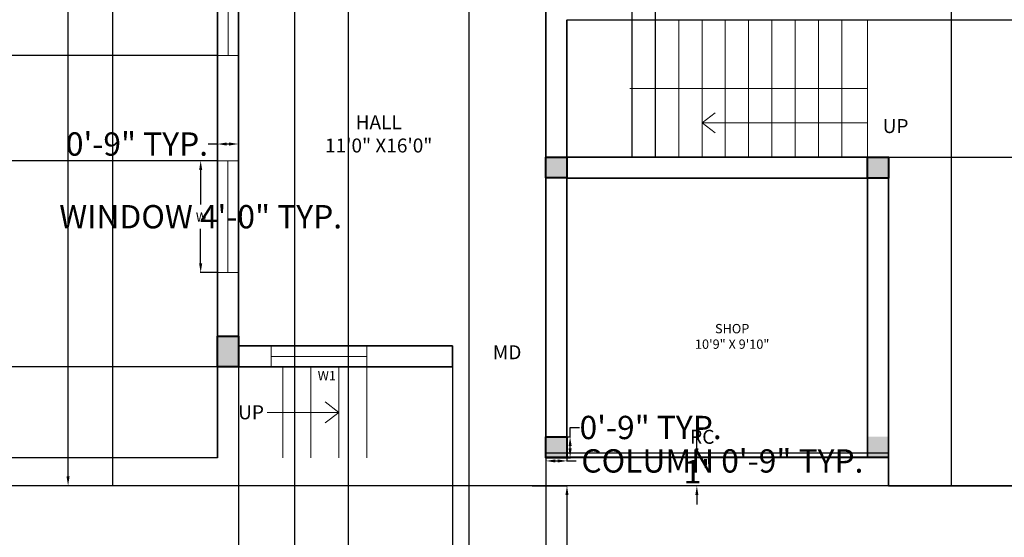
# Model space of a CAD drawing. Units: inches. Extents: x 529 to 1659, y 271 to 1222.
# Tile 3 of 5: x 936 to 1358, y 664 to 886. Entities that reach past the tile are written whole.
import ezdxf

# ---------------------------------------------------------------- set-up
doc = ezdxf.new("R2010")
doc.units = ezdxf.units.IN
doc.header["$MEASUREMENT"] = 0
for name, color, linetype, lineweight in [('A-AREA-IDEN', 7, 'Continuous', 18), ('A-COLS', 7, 'Continuous', 40), ('A-COLS-PATT', 252, 'Continuous', 13), ('A-DOOR-PATT', 4, 'Continuous', 13), ('C-ROAD', 7, 'Continuous', 25), ('COMPOUND WALL', 7, 'Continuous', 25), ('DIM', 241, 'Continuous', 18), ('DOOR', 4, 'Continuous', 25), ('STAIRCASE', 132, 'Continuous', 18), ('TEXT', 131, 'Continuous', 18), ('WALL', 7, 'Continuous', 35), ('WDS', 4, 'Continuous', 18)]:
    doc.layers.add(name, color=color, linetype=linetype, lineweight=lineweight)
doc.styles.get("Standard").update_dxf_attribs({"font": 'arial.ttf', "height": 10})
doc.dimstyles.get("Standard").update_dxf_attribs({"dimtxt": 6, "dimasz": 4, "dimexe": 0.18, "dimexo": 0.0625, "dimgap": 0.09, "dimtad": 0, "dimtih": 1, "dimtoh": 1, "dimdec": 0, "dimrnd": 6, "dimzin": 0, "dimdsep": 46, "dimlunit": 3, "dimtxsty": 'Standard', "dimcen": 0.09, "dimadec": 0, "dimazin": 0, "dimtfac": 1, "dimtdec": 0, "dimtofl": 0, "dimtmove": 0, "dimatfit": 3, "dimfxl": 1, "dimtolj": 1, "dimtzin": 0, "dimarcsym": 0})

# ---------------------------------------------------------------- blocks, each defined once
blk = doc.blocks.new('*D4')
at = {"layer": 'Defpoints', "color": 0, "transparency": 16777216}
for p in [(1228.33, 697.86), (1226.27, 685.86), (1228.33, 685.86)]:
    blk.add_point(p, dxfattribs=at)
at = {"layer": 'DIM', "color": 0, "lineweight": -2, "transparency": 16777216}
for p, q in [((1226.27, 701.86), (1226.27, 705.86)), ((1228.26, 697.86), (1226.09, 697.86)), ((1228.26, 685.86), (1226.09, 685.86)), ((1226.27, 681.86), (1226.27, 677.86))]:
    blk.add_line(p, q, dxfattribs=at)
at = {"layer": 'DIM', "color": 0, "transparency": 16777216}
for points in [[(1225.6, 701.86), (1226.94, 701.86), (1226.27, 697.86)], [(1225.6, 681.86), (1226.94, 681.86), (1226.27, 685.86)]]:
    blk.add_solid(points, dxfattribs=at)
at = {"layer": 'DIM', "color": 0, "transparency": 16777216, "insert": (1226.27, 691.86), "char_height": 10, "attachment_point": 5}
blk.add_mtext("\\A1;1'", dxfattribs=at)
blk = doc.blocks.new('*D5')
at = {"layer": 'Defpoints', "color": 0, "transparency": 16777216}
for p in [(956.28, 1165.86), (975.49, 1165.86), (975.49, 685.86)]:
    blk.add_point(p, dxfattribs=at)
at = {"layer": 'DIM', "color": 0, "lineweight": -2, "transparency": 16777216}
for p, q in [((975.43, 1165.86), (956.1, 1165.86)), ((956.28, 1161.86), (956.28, 931.05)), ((956.28, 689.86), (956.28, 920.66)), ((975.43, 685.86), (956.1, 685.86))]:
    blk.add_line(p, q, dxfattribs=at)
at = {"layer": 'DIM', "color": 0, "transparency": 16777216}
for points in [[(955.61, 1161.86), (956.94, 1161.86), (956.28, 1165.86)], [(955.61, 689.86), (956.94, 689.86), (956.28, 685.86)]]:
    blk.add_solid(points, dxfattribs=at)
at = {"layer": 'DIM', "color": 0, "transparency": 16777216, "insert": (956.28, 925.86), "char_height": 10, "attachment_point": 5}
blk.add_mtext("\\A1;40'", dxfattribs=at)
blk = doc.blocks.new('*D8')
at = {"layer": 'Defpoints', "color": 0, "transparency": 16777216}
for p in [(1155.49, 685.86), (1170.49, 685.86), (1155.55, 327.24)]:
    blk.add_point(p, dxfattribs=at)
at = {"layer": 'DIM', "color": 0, "lineweight": -2, "transparency": 16777216}
for p, q in [((1155.56, 685.86), (1170.67, 685.86)), ((1170.49, 681.86), (1170.49, 511.75)), ((1170.49, 331.24), (1170.49, 501.35)), ((1155.61, 327.24), (1170.67, 327.24))]:
    blk.add_line(p, q, dxfattribs=at)
at = {"layer": 'DIM', "color": 0, "transparency": 16777216}
for points in [[(1169.83, 681.86), (1171.16, 681.86), (1170.49, 685.86)], [(1169.83, 331.24), (1171.16, 331.24), (1170.49, 327.24)]]:
    blk.add_solid(points, dxfattribs=at)
at = {"layer": 'DIM', "color": 0, "transparency": 16777216, "insert": (1170.49, 506.55), "char_height": 10, "attachment_point": 5}
blk.add_mtext("\\A1;30'", dxfattribs=at)
blk = doc.blocks.new('WIN-48IN')
for p, q in [((9, 48), (0, 48)), ((4.5, 0), (4.5, 48)), ((9, 0), (0, 0))]:
    blk.add_line(p, q)
blk = doc.blocks.new('COL-9X9IN')
blk.add_lwpolyline([(0, 9), (9, 9), (9, 0), (0, 0)], close=True)
blk = doc.blocks.new('*D17')
at = {"layer": 'Defpoints', "color": 0, "transparency": 16777216}
for p in [(1161.49, 697.86), (1170.49, 697.86), (1170.49, 696.51)]:
    blk.add_point(p, dxfattribs=at)
at = {"layer": 'DIM', "color": 0, "lineweight": -2, "transparency": 16777216}
for p, q in [((1161.49, 697.79), (1161.49, 696.33)), ((1170.49, 697.79), (1170.49, 696.33)), ((1165.49, 696.51), (1166.49, 696.51)), ((1170.49, 696.51), (1174.49, 696.51))]:
    blk.add_line(p, q, dxfattribs=at)
at = {"layer": 'DIM', "color": 0, "transparency": 16777216}
for points in [[(1165.49, 697.17), (1165.49, 695.84), (1161.49, 696.51)], [(1166.49, 697.17), (1166.49, 695.84), (1170.49, 696.51)]]:
    blk.add_solid(points, dxfattribs=at)
at = {"layer": 'DIM', "color": 0, "transparency": 16777216, "insert": (1237.21, 696.51), "char_height": 10, "attachment_point": 5}
blk.add_mtext('\\A1;COLUMN 0\'-9" TYP.', dxfattribs=at)
blk = doc.blocks.new('*D18')
at = {"layer": 'Defpoints', "color": 0, "transparency": 16777216}
for p in [(1170.49, 706.86), (1171.84, 706.86), (1170.49, 697.86)]:
    blk.add_point(p, dxfattribs=at)
at = {"layer": 'DIM', "color": 0, "lineweight": -2, "transparency": 16777216}
for p, q in [((1171.84, 706.86), (1171.84, 710.86)), ((1171.84, 710.86), (1175.84, 710.86)), ((1170.56, 706.86), (1172.02, 706.86)), ((1171.84, 701.86), (1171.84, 702.86)), ((1170.56, 697.86), (1172.02, 697.86))]:
    blk.add_line(p, q, dxfattribs=at)
at = {"layer": 'DIM', "color": 0, "transparency": 16777216}
for points in [[(1171.18, 702.86), (1172.51, 702.86), (1171.84, 706.86)], [(1171.18, 701.86), (1172.51, 701.86), (1171.84, 697.86)]]:
    blk.add_solid(points, dxfattribs=at)
at = {"layer": 'DIM', "color": 0, "transparency": 16777216, "insert": (1206.41, 710.86), "char_height": 10, "attachment_point": 5}
blk.add_mtext('\\A1;0\'-9" TYP.', dxfattribs=at)
blk = doc.blocks.new('*D21')
at = {"layer": 'Defpoints', "color": 0, "transparency": 16777216}
for p in [(1020.41, 825.31), (1013.21, 777.31), (1020.41, 777.31)]:
    blk.add_point(p, dxfattribs=at)
at = {"layer": 'DIM', "color": 0, "lineweight": -2, "transparency": 16777216}
for p, q in [((1020.35, 825.31), (1013.03, 825.31)), ((1013.21, 821.31), (1013.21, 806.57)), ((1013.21, 781.31), (1013.21, 796.04)), ((1020.35, 777.31), (1013.03, 777.31))]:
    blk.add_line(p, q, dxfattribs=at)
at = {"layer": 'DIM', "color": 0, "transparency": 16777216}
for points in [[(1012.55, 821.31), (1013.88, 821.31), (1013.21, 825.31)], [(1012.55, 781.31), (1013.88, 781.31), (1013.21, 777.31)]]:
    blk.add_solid(points, dxfattribs=at)
at = {"layer": 'DIM', "color": 0, "transparency": 16777216, "insert": (1013.21, 801.31), "char_height": 10, "attachment_point": 5}
blk.add_mtext('\\A1;WINDOW 4\'-0" TYP.', dxfattribs=at)
blk = doc.blocks.new('*D22')
at = {"layer": 'Defpoints', "color": 0, "transparency": 16777216}
for p in [(1020.41, 832.51), (1020.41, 825.31), (1029.41, 825.31)]:
    blk.add_point(p, dxfattribs=at)
at = {"layer": 'DIM', "color": 0, "lineweight": -2, "transparency": 16777216}
for p, q in [((1020.41, 832.51), (1016.41, 832.51)), ((1020.41, 825.37), (1020.41, 832.69)), ((1025.41, 832.51), (1024.41, 832.51)), ((1029.41, 825.37), (1029.41, 832.69))]:
    blk.add_line(p, q, dxfattribs=at)
at = {"layer": 'DIM', "color": 0, "transparency": 16777216}
for points in [[(1024.41, 833.17), (1024.41, 831.84), (1020.41, 832.51)], [(1025.41, 833.17), (1025.41, 831.84), (1029.41, 832.51)]]:
    blk.add_solid(points, dxfattribs=at)
at = {"layer": 'DIM', "color": 0, "transparency": 16777216, "insert": (985.85, 832.51), "char_height": 10, "attachment_point": 5}
blk.add_mtext('\\A1;0\'-9" TYP.', dxfattribs=at)
blk = doc.blocks.new('*D28')
at = {"layer": 'Defpoints', "color": 0, "transparency": 16777216}
for p in [(1308.49, 1135.86), (1630, 1135.86), (1308.49, 685.86)]:
    blk.add_point(p, dxfattribs=at)
at = {"layer": 'DIM', "color": 0, "lineweight": -2, "transparency": 16777216}
for p, q in [((1308.56, 1135.86), (1630.18, 1135.86)), ((1630, 1131.86), (1630, 916.05)), ((1630, 689.86), (1630, 905.66)), ((1308.56, 685.86), (1630.18, 685.86))]:
    blk.add_line(p, q, dxfattribs=at)
at = {"layer": 'DIM', "color": 0, "transparency": 16777216}
for points in [[(1629.34, 1131.86), (1630.67, 1131.86), (1630, 1135.86)], [(1629.34, 689.86), (1630.67, 689.86), (1630, 685.86)]]:
    blk.add_solid(points, dxfattribs=at)
at = {"layer": 'DIM', "color": 0, "transparency": 16777216, "insert": (1630, 910.86), "char_height": 10, "attachment_point": 5}
blk.add_mtext('\\A1;37\'-6"', dxfattribs=at)
blk = doc.blocks.new('*D29')
at = {"layer": 'Defpoints', "color": 0, "transparency": 16777216}
for p in [(1076.49, 941.86), (1128.41, 941.86), (1128.41, 277.14)]:
    blk.add_point(p, dxfattribs=at)
at = {"layer": 'DIM', "color": 0, "lineweight": -2, "transparency": 16777216}
for p, q in [((1076.49, 941.79), (1076.49, 276.96)), ((1128.41, 941.79), (1128.41, 276.96)), ((1080.49, 277.14), (1088.87, 277.14)), ((1124.41, 277.14), (1116.04, 277.14))]:
    blk.add_line(p, q, dxfattribs=at)
at = {"layer": 'DIM', "color": 0, "transparency": 16777216}
for points in [[(1080.49, 277.81), (1080.49, 276.47), (1076.49, 277.14)], [(1124.41, 277.81), (1124.41, 276.47), (1128.41, 277.14)]]:
    blk.add_solid(points, dxfattribs=at)
at = {"layer": 'DIM', "color": 0, "transparency": 16777216, "insert": (1102.45, 277.14), "char_height": 10, "attachment_point": 5}
blk.add_mtext('\\A1;4\'-4"', dxfattribs=at)
blk = doc.blocks.new('*D30')
at = {"layer": 'Defpoints', "color": 0, "transparency": 16777216}
for p in [(1170.49, 885.86), (1630, 885.86), (1170.49, 826.86)]:
    blk.add_point(p, dxfattribs=at)
at = {"layer": 'DIM', "color": 0, "lineweight": -2, "transparency": 16777216}
for p, q in [((1170.56, 885.86), (1630.18, 885.86)), ((1630, 881.86), (1630, 861.47)), ((1630, 830.86), (1630, 851.24)), ((1170.56, 826.86), (1630.18, 826.86))]:
    blk.add_line(p, q, dxfattribs=at)
at = {"layer": 'DIM', "color": 0, "transparency": 16777216}
for points in [[(1629.34, 881.86), (1630.67, 881.86), (1630, 885.86)], [(1629.34, 830.86), (1630.67, 830.86), (1630, 826.86)]]:
    blk.add_solid(points, dxfattribs=at)
at = {"layer": 'DIM', "color": 0, "transparency": 16777216, "insert": (1630, 856.36), "char_height": 10, "attachment_point": 5}
blk.add_mtext('\\A1;4\'-11"', dxfattribs=at)
blk = doc.blocks.new('*D31')
at = {"layer": 'Defpoints', "color": 0, "transparency": 16777216}
for p in [(1121.32, 736.86), (1161.49, 736.86), (1161.49, 277.14)]:
    blk.add_point(p, dxfattribs=at)
at = {"layer": 'DIM', "color": 0, "lineweight": -2, "transparency": 16777216}
for p, q in [((1121.32, 736.79), (1121.32, 276.96)), ((1161.49, 736.79), (1161.49, 276.96)), ((1125.32, 277.14), (1128.03, 277.14)), ((1157.49, 277.14), (1154.78, 277.14))]:
    blk.add_line(p, q, dxfattribs=at)
at = {"layer": 'DIM', "color": 0, "transparency": 16777216}
for points in [[(1125.32, 277.81), (1125.32, 276.47), (1121.32, 277.14)], [(1157.49, 277.81), (1157.49, 276.47), (1161.49, 277.14)]]:
    blk.add_solid(points, dxfattribs=at)
at = {"layer": 'DIM', "color": 0, "transparency": 16777216, "insert": (1141.41, 277.14), "char_height": 10, "attachment_point": 5}
blk.add_mtext('\\A1;3\'-4"', dxfattribs=at)
blk = doc.blocks.new('*D32')
at = {"layer": 'Defpoints', "color": 0, "transparency": 16777216}
for p in [(555.49, 736.86), (1020.49, 736.86), (1020.49, 697.86)]:
    blk.add_point(p, dxfattribs=at)
at = {"layer": 'DIM', "color": 0, "lineweight": -2, "transparency": 16777216}
for p, q in [((1020.43, 736.86), (555.31, 736.86)), ((555.49, 732.86), (555.49, 722.55)), ((555.49, 701.86), (555.49, 712.16)), ((1020.43, 697.86), (555.31, 697.86))]:
    blk.add_line(p, q, dxfattribs=at)
at = {"layer": 'DIM', "color": 0, "transparency": 16777216}
for points in [[(554.83, 732.86), (556.16, 732.86), (555.49, 736.86)], [(554.83, 701.86), (556.16, 701.86), (555.49, 697.86)]]:
    blk.add_solid(points, dxfattribs=at)
at = {"layer": 'DIM', "color": 0, "transparency": 16777216, "insert": (555.49, 717.36), "char_height": 10, "attachment_point": 5}
blk.add_mtext('\\A1;3\'-3"', dxfattribs=at)
blk = doc.blocks.new('*D33')
at = {"layer": 'Defpoints', "color": 0, "transparency": 16777216}
for p in [(555.49, 870.44), (1020.49, 870.44), (1020.41, 825.31)]:
    blk.add_point(p, dxfattribs=at)
at = {"layer": 'DIM', "color": 0, "lineweight": -2, "transparency": 16777216}
for p, q in [((1020.43, 870.44), (555.31, 870.44)), ((555.49, 866.44), (555.49, 853.07)), ((555.49, 829.31), (555.49, 842.67)), ((1020.35, 825.31), (555.31, 825.31))]:
    blk.add_line(p, q, dxfattribs=at)
at = {"layer": 'DIM', "color": 0, "transparency": 16777216}
for points in [[(554.83, 866.44), (556.16, 866.44), (555.49, 870.44)], [(554.83, 829.31), (556.16, 829.31), (555.49, 825.31)]]:
    blk.add_solid(points, dxfattribs=at)
at = {"layer": 'DIM', "color": 0, "transparency": 16777216, "insert": (555.49, 847.87), "char_height": 10, "attachment_point": 5}
blk.add_mtext('\\A1;3\'-9"', dxfattribs=at)
blk = doc.blocks.new('*D36')
at = {"layer": 'Defpoints', "color": 0, "transparency": 16777216}
for p in [(1029.49, 1126.86), (1053.49, 1102.86), (1053.49, 277.14)]:
    blk.add_point(p, dxfattribs=at)
at = {"layer": 'DIM', "color": 0, "lineweight": -2, "transparency": 16777216}
for p, q in [((1029.49, 1126.79), (1029.49, 276.96)), ((1053.49, 1102.79), (1053.49, 276.96)), ((1033.49, 277.14), (1049.49, 277.14)), ((1053.49, 277.14), (1057.49, 277.14))]:
    blk.add_line(p, q, dxfattribs=at)
at = {"layer": 'DIM', "color": 0, "transparency": 16777216}
for points in [[(1033.49, 277.81), (1033.49, 276.47), (1029.49, 277.14)], [(1049.49, 277.81), (1049.49, 276.47), (1053.49, 277.14)]]:
    blk.add_solid(points, dxfattribs=at)
at = {"layer": 'DIM', "color": 0, "transparency": 16777216, "insert": (1070.96, 277.14), "char_height": 10, "attachment_point": 5}
blk.add_mtext('\\A1;2\'-0"', dxfattribs=at)
blk = doc.blocks.new('*D37')
at = {"layer": 'Defpoints', "color": 0, "transparency": 16777216}
for p in [(1208.47, 1214.96), (1198.47, 826.86), (1208.47, 826.86)]:
    blk.add_point(p, dxfattribs=at)
at = {"layer": 'DIM', "color": 0, "lineweight": -2, "transparency": 16777216}
for p, q in [((1198.47, 826.92), (1198.47, 1215.14)), ((1202.47, 1214.96), (1204.47, 1214.96)), ((1208.47, 826.92), (1208.47, 1215.14)), ((1208.47, 1214.96), (1212.47, 1214.96))]:
    blk.add_line(p, q, dxfattribs=at)
at = {"layer": 'DIM', "color": 0, "transparency": 16777216}
for points in [[(1202.47, 1215.62), (1202.47, 1214.29), (1198.47, 1214.96)], [(1204.47, 1215.62), (1204.47, 1214.29), (1208.47, 1214.96)]]:
    blk.add_solid(points, dxfattribs=at)
at = {"layer": 'DIM', "color": 0, "transparency": 16777216, "insert": (1229.74, 1214.96), "char_height": 10, "attachment_point": 5}
blk.add_mtext('\\A1;0\'-10"', dxfattribs=at)

msp = doc.modelspace()

# ---------------------------------------------------------------- hatches: boundary and pattern name
at = {"layer": 'A-COLS-PATT'}
h = msp.add_hatch(color=256, dxfattribs=at)
h.dxf.hatch_style = 1
h.paths.add_polyline_path([(1169.49, 1135.86), (1159.82, 1135.86), (1159.82, 1125.57), (1169.49, 1125.57), (1169.49, 1126.86)])
h.paths.add_polyline_path([(1308.49, 1135.86), (1299.49, 1135.86), (1299.49, 1126.86), (1308.49, 1126.86)])
h.paths.add_polyline_path([(1029.49, 1135.86), (1020.49, 1135.86), (1020.49, 1122.62), (1029.49, 1122.62)])
h.paths.add_polyline_path([(1029.49, 941.86), (1020.49, 941.86), (1020.49, 931.16), (1029.49, 931.16)])
h.paths.add_polyline_path([(1170.49, 941.72), (1161.49, 941.72), (1161.49, 932.72), (1170.49, 932.72)])
h.paths.add_polyline_path([(1308.49, 941.86), (1299.49, 941.86), (1299.49, 928.64), (1308.49, 928.64)])
h.paths.add_polyline_path([(1308.49, 826.86), (1299.49, 826.86), (1299.49, 817.86), (1308.49, 817.86)])
h.paths.add_polyline_path([(1170.49, 826.93), (1161.49, 826.93), (1161.49, 817.93), (1170.49, 817.93)])
h.paths.add_polyline_path([(1308.49, 706.86), (1299.49, 706.86), (1299.49, 697.86), (1308.49, 697.86)])
h.paths.add_polyline_path([(1170.49, 706.86), (1161.49, 706.86), (1161.49, 697.86), (1170.49, 697.86)])
h.paths.add_polyline_path([(1029.41, 750.01), (1020.49, 750.01), (1020.49, 736.86), (1029.49, 736.86)])
at = {"layer": 'A-DOOR-PATT'}
h = msp.add_hatch(dxfattribs=at)
h.set_pattern_fill('ANSI31', color=256, scale=0.8, angle=-45, style=0)
h.paths.add_polyline_path([(1161.49, 697.86), (1308.49, 697.86), (1308.49, 698.36), (1161.49, 698.36)])

# ---------------------------------------------------------------- linework, layer by layer
at = {"layer": 'A-COLS'}
for p, q in [((1020.41, 750.01), (1029.41, 750.01)), ((1020.49, 736.86), (1020.41, 750.01)), ((1029.41, 750.01), (1029.49, 736.86)), ((1029.49, 736.86), (1020.49, 736.86))]:
    msp.add_line(p, q, dxfattribs=at)
at = {"layer": 'C-ROAD'}
msp.add_line((1567.16, 685.86), (618.33, 685.86), dxfattribs=at)
msp.add_line((1567.16, 685.86), (618.33, 685.86), dxfattribs=at)
at = {"layer": 'COMPOUND WALL'}
for p, q in [((975.49, 685.86), (975.49, 1165.86)), ((1335.49, 1165.86), (1335.49, 685.86)), ((1335.49, 685.86), (975.49, 685.86))]:
    msp.add_line(p, q, dxfattribs=at)
at = {"layer": 'DOOR'}
for p, q in [((1308.49, 699.86), (1161.49, 699.86)), ((1161.49, 697.86), (1161.49, 698.36))]:
    msp.add_line(p, q, dxfattribs=at)
at = {"layer": 'STAIRCASE'}
for p, q in [((1198.47, 885.86), (1198.47, 826.86)), ((1208.47, 885.86), (1208.47, 826.86)), ((1218.48, 885.86), (1218.48, 826.86)), ((1228.48, 885.86), (1228.48, 826.86)), ((1238.48, 885.86), (1238.48, 826.86)), ((1248.48, 885.86), (1248.48, 826.86)), ((1258.49, 885.86), (1258.49, 826.86)), ((1268.49, 885.86), (1268.49, 826.86)), ((1278.49, 885.86), (1278.49, 826.86)), ((1288.49, 885.86), (1288.49, 826.86)), ((1299.49, 885.86), (1299.49, 826.86)), ((1299.49, 856.36), (1197.47, 856.36)), ((1228.48, 841.61), (1234.14, 845.92)), ((1299.49, 841.61), (1228.48, 841.61)), ((1228.48, 841.61), (1234.14, 837.29)), ((1048.49, 697.86), (1048.49, 736.86)), ((1060.49, 697.86), (1060.49, 736.86)), ((1072.49, 697.86), (1072.49, 736.86)), ((1084.49, 697.86), (1084.49, 736.86)), ((1072.49, 717.36), (1066.69, 721.89)), ((1041.72, 717.36), (1072.49, 717.36)), ((1072.49, 717.36), (1066.69, 712.82))]:
    msp.add_line(p, q, dxfattribs=at)
at = {"layer": 'WALL'}
for p, q in [((1020.49, 697.86), (1020.49, 1135.86)), ((1029.49, 736.86), (1029.49, 980.86)), ((1161.49, 736.86), (1161.49, 941.86)), ((1170.49, 826.86), (1170.49, 885.86)), ((1308.49, 826.86), (1170.49, 826.86)), ((1308.49, 826.86), (1308.49, 685.86)), ((1308.49, 826.86), (1308.49, 685.86)), ((1170.49, 697.86), (1170.49, 817.86)), ((1299.49, 817.86), (1170.49, 817.86)), ((1299.49, 817.86), (1299.49, 697.86)), ((1029.49, 745.86), (1121.32, 745.86)), ((1121.32, 736.86), (1121.32, 745.86)), ((1020.49, 736.86), (1121.32, 736.86)), ((1161.49, 697.86), (1161.49, 736.86))]:
    msp.add_line(p, q, dxfattribs=at)
at = {"layer": 'WDS'}
for p, q in [((1043.5, 736.86), (1043.5, 745.86)), ((1084.49, 736.86), (1084.49, 745.86)), ((1084.49, 741.36), (1043.5, 741.36))]:
    msp.add_line(p, q, dxfattribs=at)

# ---------------------------------------------------------------- block references
at = {"layer": 'A-COLS'}
for p in [(1161.49, 817.93), (1299.49, 817.85), (1161.49, 697.86)]:
    msp.add_blockref('COL-9X9IN', p, dxfattribs=at)
at = {"layer": 'WDS'}
msp.add_blockref('WIN-48IN', (1020.49, 870.43), dxfattribs=at)
at = {"layer": 'WDS', "rotation": 180}
msp.add_blockref('WIN-48IN', (1029.41, 825.31), dxfattribs=at)

# ---------------------------------------------------------------- texts
at = {"layer": 'A-AREA-IDEN', "attachment_point": 1}
for s, width, insert, char_height in [('\\pxqc;HALL\\P11\'0" X16\'0"', 59.3536, (1059.97, 844.87), 6), ('\\pxqc;SHOP\\P10\'9" X 9\'10"', 41.7934, (1220.53, 755.28), 4)]:
    msp.add_mtext_dynamic_manual_height_columns(s, width=width, gutter_width=20, heights=[0], dxfattribs=dict(at, insert=insert, char_height=char_height))
at = {"layer": 'TEXT', "attachment_point": 1}
for s, width, gutter_width, insert, char_height in [('\\pxqc;UP', 16.0307, 20, (1303.57, 843.22), 6), ('W ', 22.0133, 20, (1011.14, 803.17), 4), ('\\pxqc;MD', 21.6865, 20, (1133.96, 746.13), 6), ('W1 ', 22.0133, 20, (1063.46, 735.06), 4), ('\\pxqc;UP', 12.7261, 20, (1028.48, 720.37), 6), ('RC', 37.456, 50, (1223.38, 709.86), 6)]:
    msp.add_mtext_dynamic_manual_height_columns(s, width=width, gutter_width=gutter_width, heights=[0], dxfattribs=dict(at, insert=insert, char_height=char_height))

# ---------------------------------------------------------------- dimensions: what is measured, and where the dimension line sits
at = {"layer": 'DIM'}
for base, p1, p2, picture, middle in [((1208.47, 1214.96), (1198.47, 826.86), (1208.47, 826.86), '*D37', (1229.74, 1214.96)), ((1053.49, 277.14), (1029.49, 1126.86), (1053.49, 1102.86), '*D36', (1070.96, 277.14)), ((1128.41, 277.14), (1076.49, 941.86), (1128.41, 941.86), '*D29', (1102.45, 277.14)), ((1161.49, 277.14), (1121.32, 736.86), (1161.49, 736.86), '*D31', (1141.41, 277.14))]:
    dim = msp.add_linear_dim(base=base, p1=p1, p2=p2, dimstyle='Standard', override={"dimdec": 1, "dimlfac": 1, "dimrnd": 0, "dimzin": 1, "dimdsep": 46, "dimlunit": 4, "dimfrac": 2}, dxfattribs=at)
    dim.commit()
    dim.dimension.update_dxf_attribs({"geometry": picture, "text_midpoint": middle})
for base, p1, p2, override, picture, middle in [((956.28, 1165.86), (975.49, 685.86), (975.49, 1165.86), {"dimclrd": 0, "dimclre": 0, "dimclrt": 0}, '*D5', (956.28, 925.86)), ((1630, 1135.86), (1308.49, 685.86), (1308.49, 1135.86), {"dimdec": 1, "dimlfac": 1, "dimrnd": 0, "dimzin": 1, "dimdsep": 46, "dimlunit": 4, "dimfrac": 2}, '*D28', (1630, 910.86)), ((1630, 885.86), (1170.49, 826.86), (1170.49, 885.86), {"dimdec": 1, "dimlfac": 1, "dimrnd": 0, "dimzin": 1, "dimdsep": 46, "dimlunit": 4, "dimfrac": 2}, '*D30', (1630, 856.36)), ((555.49, 870.44), (1020.41, 825.31), (1020.49, 870.44), {"dimdec": 1, "dimlfac": 1, "dimrnd": 0, "dimzin": 1, "dimdsep": 46, "dimlunit": 4, "dimfrac": 2}, '*D33', (555.49, 847.87)), ((555.49, 736.86), (1020.49, 697.86), (1020.49, 736.86), {"dimdec": 1, "dimlfac": 1, "dimrnd": 0, "dimzin": 1, "dimdsep": 46, "dimlunit": 4, "dimfrac": 2}, '*D32', (555.49, 717.36)), ((1226.27, 685.86), (1228.33, 697.86), (1228.33, 685.86), {"dimclrd": 0, "dimclre": 0, "dimclrt": 0}, '*D4', (1226.27, 691.86)), ((1170.49, 685.86), (1155.55, 327.24), (1155.49, 685.86), {"dimclrd": 0, "dimclre": 0, "dimclrt": 0}, '*D8', (1170.49, 506.55))]:
    dim = msp.add_linear_dim(base=base, p1=p1, p2=p2, angle=90, dimstyle='Standard', override=override, dxfattribs=at)
    dim.commit()
    dim.dimension.update_dxf_attribs({"geometry": picture, "text_midpoint": middle})
for base, p1, p2, angle, text, picture, middle in [((1020.41, 832.51), (1029.41, 825.31), (1020.41, 825.31), 180, '<> TYP.', '*D22', (985.85, 832.51)), ((1013.21, 777.31), (1020.41, 825.31), (1020.41, 777.31), 270, 'WINDOW <> TYP.', '*D21', (1013.21, 801.31)), ((1171.84, 706.86), (1170.49, 697.86), (1170.49, 706.86), 90, '<> TYP.', '*D18', (1206.41, 710.86))]:
    dim = msp.add_linear_dim(base=base, p1=p1, p2=p2, angle=angle, text=text, dimstyle='Standard', override={"dimdec": 1, "dimlfac": 1, "dimrnd": 0, "dimzin": 1, "dimdsep": 46, "dimlunit": 4, "dimfrac": 2}, dxfattribs=at)
    dim.commit()
    dim.dimension.update_dxf_attribs({"geometry": picture, "text_midpoint": middle})
dim = msp.add_linear_dim(base=(1170.49, 696.51), p1=(1161.49, 697.86), p2=(1170.49, 697.86), text='COLUMN <> TYP.', dimstyle='Standard', override={"dimdec": 1, "dimlfac": 1, "dimrnd": 0, "dimzin": 1, "dimdsep": 46, "dimlunit": 4, "dimfrac": 2}, dxfattribs=at)
dim.commit()
dim.dimension.update_dxf_attribs({"geometry": '*D17', "text_midpoint": (1237.21, 696.51)})

doc.saveas('drawing.dxf')
